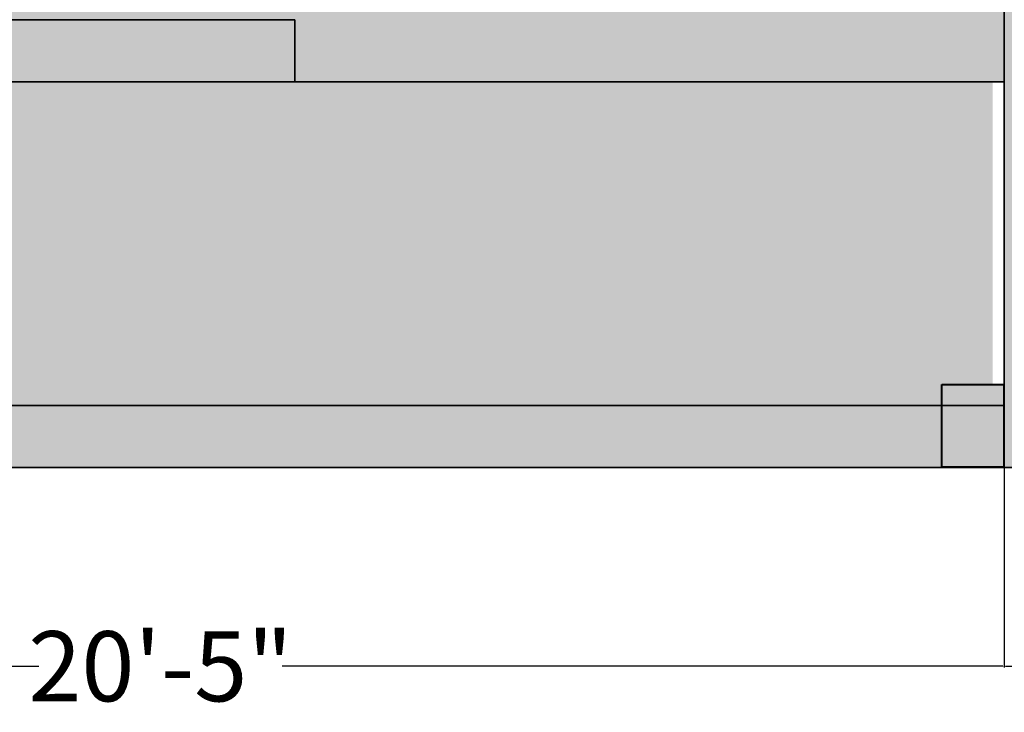
# Model space of a CAD drawing. Units: inches. Extents: x 1077 to 2505, y 1892 to 2728.
# Tile 4 of 26: x 1290 to 1433, y 2053 to 2153. Entities that reach past the tile are written whole.
import ezdxf

# ---------------------------------------------------------------- set-up
doc = ezdxf.new("R2010")
doc.units = ezdxf.units.IN
doc.linetypes.add('ACAD_ISO02W100', pattern=[15, 12, -3])
doc.layers.get('Defpoints').update_dxf_attribs({"color": 220, "linetype": 'ACAD_ISO02W100'})
for name, color, linetype, lineweight in [('A-ANNO-DIMS', 2, 'Continuous', 18), ('A-COLS', 7, 'Continuous', 40), ('A-WALL-PATT', 7, 'Continuous', 9), ('WALL', 7, 'Continuous', 35)]:
    doc.layers.add(name, color=color, linetype=linetype, lineweight=lineweight)
doc.layers.add('A-FLOR-PATT', color=254, linetype='Continuous', lineweight=9, true_color=0xd7ebd2)
doc.layers.add('L-PLNT-PATT', color=116, linetype='Continuous', lineweight=9, true_color=0x136734)
doc.styles.get("Standard").update_dxf_attribs({"font": 'arial.ttf'})
doc.dimstyles.get("Standard").update_dxf_attribs({"dimtxt": 10.18, "dimasz": 0.18, "dimexe": 0.18, "dimexo": 0.0625, "dimgap": 0.09, "dimtad": 0, "dimtih": 1, "dimtoh": 1, "dimdec": 0, "dimzin": 0, "dimdsep": 46, "dimlunit": 3, "dimtxsty": 'Standard', "dimcen": 0.09, "dimadec": 0, "dimazin": 0, "dimtfac": 1, "dimtdec": 0, "dimtofl": 0, "dimtmove": 0, "dimatfit": 3, "dimfxl": 1, "dimtolj": 1, "dimtzin": 0, "dimarcsym": 0})

# ---------------------------------------------------------------- blocks, each defined once
blk = doc.blocks.new('C1')
h = blk.add_hatch(color=256)
h.dxf.hatch_style = 1
h.paths.add_polyline_path([(1668.56, 2445.41), (1677.56, 2445.41), (1677.56, 2457.41), (1668.56, 2457.41)])
for p, q in [((1668.56, 2457.41), (1677.56, 2457.41)), ((1668.56, 2445.41), (1668.56, 2457.41)), ((1677.56, 2457.41), (1677.56, 2445.41)), ((1677.56, 2445.41), (1668.56, 2445.41))]:
    blk.add_line(p, q)
blk = doc.blocks.new('*D65')
at = {"layer": 'A-ANNO-DIMS', "color": 0, "lineweight": -2, "transparency": 16777216}
for p, q in [((1187.53, 2097.1), (1187.53, 2059.13)), ((1432.53, 2097.1), (1432.53, 2059.13)), ((1187.71, 2059.31), (1292.37, 2059.31)), ((1432.35, 2059.31), (1327.69, 2059.31))]:
    blk.add_line(p, q, dxfattribs=at)
at = {"layer": 'A-ANNO-DIMS', "color": 0, "transparency": 16777216}
for points in [[(1187.71, 2059.34), (1187.71, 2059.28), (1187.53, 2059.31)], [(1432.35, 2059.34), (1432.35, 2059.28), (1432.53, 2059.31)]]:
    blk.add_solid(points, dxfattribs=at)
at = {"layer": 'Defpoints', "color": 0, "transparency": 16777216}
for p in [(1187.53, 2097.16), (1432.53, 2097.16), (1432.53, 2059.31)]:
    blk.add_point(p, dxfattribs=at)
at = {"layer": 'A-ANNO-DIMS', "color": 0, "transparency": 16777216, "insert": (1310.03, 2059.31), "char_height": 10.18, "attachment_point": 5}
blk.add_mtext('\\A1;20\'-5"', dxfattribs=at)
blk = doc.blocks.new('*D67')
at = {"layer": 'A-ANNO-DIMS', "color": 0, "lineweight": -2, "transparency": 16777216}
for p, q in [((1432.53, 2088.1), (1432.53, 2059.13)), ((1547.53, 2088.1), (1547.53, 2059.13)), ((1432.71, 2059.31), (1476.41, 2059.31)), ((1547.35, 2059.31), (1503.65, 2059.31))]:
    blk.add_line(p, q, dxfattribs=at)
at = {"layer": 'A-ANNO-DIMS', "color": 0, "transparency": 16777216}
for points in [[(1432.71, 2059.34), (1432.71, 2059.28), (1432.53, 2059.31)], [(1547.35, 2059.34), (1547.35, 2059.28), (1547.53, 2059.31)]]:
    blk.add_solid(points, dxfattribs=at)
at = {"layer": 'Defpoints', "color": 0, "transparency": 16777216}
for p in [(1432.53, 2088.16), (1547.53, 2088.16), (1547.53, 2059.31)]:
    blk.add_point(p, dxfattribs=at)
at = {"layer": 'A-ANNO-DIMS', "color": 0, "transparency": 16777216, "insert": (1490.03, 2059.31), "char_height": 10.18, "attachment_point": 5}
blk.add_mtext('\\A1;9\'-7"', dxfattribs=at)

msp = doc.modelspace()

# ---------------------------------------------------------------- hatches: boundary and pattern name
at = {"layer": 'A-FLOR-PATT', "transparency": 33554559}
h = msp.add_hatch(color=256, dxfattribs=at)
h.dxf.hatch_style = 1
h.paths.add_polyline_path([(1395.53, 2577.16), (1374.83, 2577.16), (1350.83, 2577.19), (1350.83, 2577.16), (1329.53, 2577.16), (1329.53, 2480.16), (1329.53, 2469.16), (1325.53, 2469.16), (1325.53, 2515.13), (1307.53, 2515.13), (1307.53, 2577.16), (1269.31, 2577.16), (1221.31, 2577.15), (1221.31, 2577.16), (1187.53, 2577.16), (1187.53, 2433.16), (1289.53, 2433.16), (1289.53, 2429.16), (1263.53, 2429.16), (1187.53, 2429.16), (1187.53, 2395.02), (1187.53, 2395.02), (1187.53, 2371.02), (1187.53, 2371.02), (1187.53, 2307.16), (1259.53, 2307.16), (1259.53, 2399.16), (1263.53, 2399.16), (1263.53, 2307.16), (1289.53, 2307.16), (1289.53, 2306.23), (1325.53, 2306.23), (1325.53, 2307.16), (1329.53, 2307.16), (1329.53, 2306.23), (1365.53, 2306.23), (1365.53, 2307.16), (1432.53, 2307.16), (1432.53, 2088.16), (1547.53, 2088.16), (1547.53, 2140.08), (1511.53, 2140.08), (1511.53, 2267.16), (1475.53, 2267.16), (1475.53, 2303.16), (1468.53, 2303.16), (1468.53, 2307.16), (1547.53, 2307.16), (1547.53, 2348.22), (1547.53, 2396.22), (1547.53, 2429.16), (1435.53, 2429.16), (1435.53, 2433.16), (1476.35, 2433.16), (1476.35, 2451.18), (1547.53, 2451.18), (1547.53, 2577.16), (1499.53, 2577.16), (1499.53, 2586.16), (1547.53, 2586.16), (1547.53, 2642.16), (1518.18, 2642.16), (1518.18, 2642.05), (1494.15, 2642.05), (1494.15, 2642.16), (1469.53, 2642.16), (1469.53, 2577.16), (1399.53, 2577.16), (1399.53, 2429.16), (1325.53, 2429.16), (1325.53, 2433.16), (1329.53, 2433.16), (1395.53, 2433.16), (1395.53, 2480.16), (1359.53, 2480.16), (1359.53, 2484.16), (1395.53, 2484.16)])
h.paths.add_polyline_path([(1357.65, 2482.07), (1355.65, 2482.07), (1355.65, 2481.07, 0.414214), (1356.65, 2480.07), (1344.65, 2480.07), (1344.65, 2477.06), (1343.27, 2477.06), (1343.27, 2480.07), (1330.65, 2480.07, -0.414214), (1329.65, 2481.07), (1329.65, 2484.07), (1331.65, 2484.07), (1331.65, 2510.07, -0.446908)], flags=16)
h.paths.add_polyline_path([(1305.09, 2559.18), (1288.89, 2559.18), (1288.89, 2575.38), (1305.09, 2575.38)], flags=16)
h.paths.add_polyline_path([(1304.19, 2560.08), (1289.79, 2560.08), (1289.79, 2574.48), (1304.19, 2574.48)], flags=0)
h.paths.add_polyline_path([(1287.99, 2500.68, -0.414214), (1287.09, 2499.78), (1265.14, 2499.78), (1224.09, 2499.78, -0.414214), (1223.19, 2500.68), (1223.19, 2557.16), (1223.19, 2571.74), (1223.19, 2575.38), (1287.99, 2575.38), (1287.99, 2571.74), (1287.09, 2571.74, -0.414214), (1287.99, 2570.84)], flags=16)
h.paths.add_polyline_path([(1292.98, 2569.05, -1), (1300.92, 2569.05, -1)], flags=0)
h.paths.add_polyline_path([(1293.32, 2569.05, -1), (1300.58, 2569.05, -1)], flags=0)
h.paths.add_polyline_path([(1322.8, 2462.21), (1322.8, 2431.71), (1323.05, 2430.71), (1323.05, 2431.71), (1321.8, 2431.71), (1321.8, 2462.19, 0.404641), (1292.3, 2431.71), (1292.05, 2430.71, -0.414214), (1291.55, 2430.21), (1291.05, 2430.21), (1291.05, 2429.71, -0.414214), (1290.55, 2429.21), (1289.55, 2429.21), (1289.55, 2434.21), (1290.55, 2434.21, -0.414214), (1291.05, 2433.71), (1291.05, 2433.21), (1291.55, 2433.21, -0.414214), (1292.05, 2432.71), (1292.3, 2431.71, -0.414214)], flags=16)
h.paths.add_polyline_path([(1287.82, 2548.28, 0.292232), (1279.17, 2536.8, 0.052719), (1223.93, 2548.28), (1223.28, 2548.28), (1223.28, 2557.16), (1223.93, 2557.16), (1245.42, 2557.16, -0.117785), (1245.77, 2557.93, -0.059418), (1254.87, 2567.02, -0.379859), (1257.28, 2566.88, -0.02509), (1261.41, 2563.32, -0.025935), (1265.65, 2567.02, -0.379859), (1268.06, 2566.88, -0.061767), (1277.52, 2557.43, -0.069393), (1277.82, 2557.16), (1287.82, 2557.16)], flags=0)
h.paths.add_polyline_path([(1263.47, 2548.28), (1260.56, 2548.28, -0.015371), (1258.01, 2546.13, -0.429576), (1255.37, 2546.06, -0.016036), (1252.69, 2548.28), (1223.28, 2548.28), (1223.28, 2554.42), (1246.78, 2554.42, 0.055344), (1255.37, 2546.06, 0.331768), (1257.52, 2545.74, 0.027343), (1262, 2549.64, 0.00919)], flags=0)
h.paths.add_polyline_path([(1295.56, 2568.34), (1296.87, 2569.09), (1296.87, 2570.6, 0.399698), (1295.39, 2569.05, 0.119004)], flags=0)
h.paths.add_polyline_path([(1295.21, 2569.05, -1), (1298.68, 2569.05, -1)], flags=0)
h.paths.add_polyline_path([(1296.95, 2568.96), (1297.03, 2569), (1297.03, 2569.09), (1296.99, 2569.11), (1296.91, 2568.98)], flags=0)
h.paths.add_polyline_path([(1402.28, 2462.19, -0.414214), (1432.78, 2431.69), (1433.03, 2432.69), (1432.78, 2431.69, 0.404641), (1403.28, 2462.17), (1403.28, 2431.69), (1402.03, 2431.69), (1402.03, 2430.69, -0.414214), (1401.53, 2430.19), (1401.03, 2430.19), (1401.03, 2429.69, -0.414214), (1400.53, 2429.19), (1399.53, 2429.19), (1399.53, 2434.19), (1400.53, 2434.19, -0.414214), (1401.03, 2433.69), (1401.03, 2433.19), (1401.53, 2433.19, -0.414214), (1402.03, 2432.69)], flags=16)
h.paths.add_polyline_path([(1470.16, 2535.21, -0.414214), (1471.06, 2536.11), (1527.54, 2536.11), (1542.12, 2536.11), (1545.76, 2536.11), (1545.76, 2471.31), (1542.12, 2471.31), (1542.12, 2472.21, -0.414214), (1541.22, 2471.31), (1471.06, 2471.31, -0.414214), (1470.16, 2472.21), (1470.16, 2494.16)], flags=16)
h.paths.add_polyline_path([(1483.07, 2536.11, 0.253465), (1480.11, 2526.15, 0.2538), (1470.15, 2523.19)], flags=16)
h.paths.add_polyline_path([(1223.19, 2512.69, 0.253465), (1233.14, 2509.74, 0.2538), (1236.1, 2499.77)], flags=16)
h.paths.add_polyline_path([(1469.77, 2578.72), (1469.77, 2581.72), (1471.77, 2581.72), (1471.77, 2607.72, -0.01951), (1473.77, 2607.68), (1473.77, 2579.72), (1473.77, 2578.72, -0.414214), (1472.77, 2577.72), (1470.77, 2577.72, -0.414214)], flags=16)
h.paths.add_polyline_path([(1382.46, 2398.13), (1395.04, 2398.13), (1395.04, 2399.74), (1382.46, 2399.74)], flags=16)
h.paths.add_polyline_path([(1379.94, 2397.18), (1379.94, 2389.82), (1380.5, 2389.82), (1380.5, 2396.05, -0.41429), (1381.06, 2396.61), (1396.47, 2396.61, -0.414213), (1397.03, 2396.05), (1397.03, 2389.82), (1397.59, 2389.82), (1397.59, 2397.18)], flags=16)
h.paths.add_polyline_path([(1263.37, 2428.14), (1263.37, 2426.14, -0.414214), (1262.37, 2425.14), (1261.37, 2425.14), (1233.41, 2425.14, 0.400854), (1259.37, 2401.04), (1259.37, 2401.14), (1261.37, 2401.14, -0.446908), (1233.37, 2427.14), (1259.37, 2427.14), (1259.37, 2429.14), (1262.37, 2429.14, -0.414214)], flags=16)
h.paths.add_polyline_path([(1404.79, 2398.13), (1417.37, 2398.13), (1417.37, 2399.74), (1404.79, 2399.74)], flags=16)
h.paths.add_polyline_path([(1402.27, 2397.18), (1404.79, 2398.13), (1417.37, 2398.13), (1419.92, 2397.18)], flags=16)
h.paths.add_polyline_path([(1432.26, 2383.16), (1432.26, 2370.59), (1433.87, 2370.59), (1433.87, 2383.16)], flags=16)
h.paths.add_polyline_path([(1431.3, 2385.69), (1423.84, 2385.69), (1423.84, 2385.13), (1430.18, 2385.13, -0.41429), (1430.74, 2384.57), (1430.74, 2369.16, -0.414237), (1430.18, 2368.6), (1423.84, 2368.6), (1423.84, 2368.03), (1431.3, 2368.03)], flags=16)
h.paths.add_polyline_path([(1417.37, 2351.16), (1417.37, 2349.54), (1418.9, 2349.54, 0.414236), (1419.92, 2350.56), (1419.92, 2352.11)], flags=16)
h.paths.add_polyline_path([(1395.04, 2351.16), (1395.04, 2349.54), (1396.58, 2349.54, 0.414235), (1397.59, 2350.56), (1397.59, 2352.11)], flags=16)
h.paths.add_polyline_path([(1366.7, 2370.05), (1365.09, 2370.05), (1365.09, 2368.52, 0.414235), (1366.11, 2367.5), (1367.66, 2367.5)], flags=16)
h.paths.add_polyline_path([(1419.36, 2359.47), (1419.36, 2353.24, -0.41419), (1418.8, 2352.68), (1403.39, 2352.68, -0.414137), (1402.83, 2353.24), (1402.83, 2359.47), (1397.03, 2359.47), (1397.03, 2353.24, -0.414189), (1396.47, 2352.68), (1381.06, 2352.68, -0.414137), (1380.5, 2353.24), (1380.5, 2359.47)], flags=16)
h.paths.add_polyline_path([(1222.29, 2559.18), (1206.09, 2559.18), (1206.09, 2575.38), (1222.29, 2575.38)], flags=16)
h.paths.add_polyline_path([(1221.39, 2560.08), (1206.99, 2560.08), (1206.99, 2574.48), (1221.39, 2574.48)], flags=0)
h.paths.add_polyline_path([(1482, 2577.72), (1482, 2580.73), (1483.38, 2580.73), (1483.38, 2577.72), (1484.77, 2577.72), (1484.77, 2574.72), (1483.38, 2574.72), (1483.38, 2577.72)], flags=16)
h.paths.add_polyline_path([(1266.37, 2415.53), (1266.37, 2414.14), (1263.37, 2414.14), (1263.37, 2415.53), (1260.36, 2415.53), (1260.36, 2416.91), (1263.37, 2416.91), (1263.37, 2415.53)], flags=16)
h.paths.add_polyline_path([(1210.26, 2569.05, -1), (1218.19, 2569.05, -1)], flags=0)
h.paths.add_polyline_path([(1210.6, 2569.05, -1), (1217.85, 2569.05, -1)], flags=0)
h.paths.add_polyline_path([(1212.84, 2568.34), (1214.15, 2569.09), (1214.15, 2570.6, 0.399698), (1212.67, 2569.05, 0.119004)], flags=0)
h.paths.add_polyline_path([(1212.49, 2569.05, -1), (1215.96, 2569.05, -1)], flags=0)
h.paths.add_polyline_path([(1214.23, 2568.96), (1214.3, 2568.91), (1214.3, 2569)], flags=0)
h.paths.add_polyline_path([(1507.18, 2480.12, 0.052719), (1518.66, 2535.36), (1518.66, 2536.01), (1527.54, 2536.01), (1527.54, 2535.36), (1527.54, 2513.88, -0.117785), (1528.31, 2513.53, -0.059418), (1537.4, 2504.43, -0.379859), (1537.26, 2502.01, -0.02509), (1533.7, 2497.89, -0.025935), (1537.4, 2493.64, -0.379859), (1537.26, 2491.23, -0.061767), (1527.8, 2481.77, -0.069393), (1527.54, 2481.47), (1527.54, 2471.47), (1518.66, 2471.47, 0.292232)], flags=0)
h.paths.add_polyline_path([(1516.43, 2503.92, -0.016036), (1518.66, 2506.6), (1518.66, 2536.01), (1524.8, 2536.01), (1524.8, 2512.51, 0.055344), (1516.43, 2503.92, 0.331768), (1516.12, 2501.77, 0.027343), (1520.01, 2497.29, 0.00919), (1518.66, 2495.82), (1518.66, 2498.73, -0.015371), (1516.5, 2501.28, -0.429576)], flags=0)
h.paths.add_polyline_path([(1499.63, 2625.5, -0.171636), (1502.82, 2631.01), (1502.82, 2633.37), (1498.68, 2633.37, -0.414214), (1497.7, 2634.36), (1497.7, 2640.66, -0.414214), (1498.68, 2641.64), (1514.82, 2641.64, -0.414214), (1515.81, 2640.66), (1515.81, 2634.36, -0.414214), (1514.82, 2633.37), (1510.69, 2633.37), (1510.69, 2631.01, -0.171636), (1513.88, 2625.5, -0.258205), (1509.31, 2614.47), (1504.19, 2614.47, -0.258205)], flags=16)
h.paths.add_polyline_path([(1501.2, 2625.5, -0.171636), (1504.39, 2631.01), (1509.12, 2631.01, -0.171636), (1512.3, 2625.5, -0.210384), (1509.35, 2616.02), (1504.16, 2616.02, -0.210384)], flags=0)
h.paths.add_polyline_path([(1529.56, 2537.01), (1529.56, 2553.21), (1545.76, 2553.21), (1545.76, 2537.01)], flags=16)
h.paths.add_polyline_path([(1530.46, 2537.91), (1530.46, 2552.31), (1544.86, 2552.31), (1544.86, 2537.91)], flags=0)
h.paths.add_polyline_path([(1535.45, 2545.07, -1), (1543.39, 2545.07, -1)], flags=0)
h.paths.add_polyline_path([(1535.8, 2545.07, -1), (1543.05, 2545.07, -1)], flags=0)
h.paths.add_polyline_path([(1529.56, 2470.41), (1545.76, 2470.41), (1545.76, 2454.21), (1529.56, 2454.21)], flags=16)
h.paths.add_polyline_path([(1541.16, 2544.99), (1540.98, 2544.99, -0.544606), (1538.71, 2543.68), (1538.62, 2543.53, 0.547962)], flags=0)
h.paths.add_polyline_path([(1530.46, 2469.51), (1544.86, 2469.51), (1544.86, 2455.11), (1530.46, 2455.11)], flags=0)
h.paths.add_polyline_path([(1539.47, 2545.14), (1539.42, 2545.22), (1539.38, 2545.14)], flags=0)
h.paths.add_polyline_path([(1543.39, 2462.34, -1), (1535.45, 2462.34, -1)], flags=0)
h.paths.add_polyline_path([(1543.05, 2462.34, -1), (1535.8, 2462.34, -1)], flags=0)
h.paths.add_polyline_path([(1541.16, 2462.27), (1540.98, 2462.27, -0.544606), (1538.71, 2460.96), (1538.62, 2460.8, 0.547962)], flags=0)
h.paths.add_polyline_path([(1539.47, 2462.42), (1539.42, 2462.5), (1539.38, 2462.42)], flags=0)
h.paths.add_polyline_path([(1435.32, 2335.25, -0.414214), (1465.82, 2304.75), (1466.07, 2305.75), (1465.82, 2304.75, 0.404641), (1436.32, 2335.23), (1436.32, 2304.75), (1435.07, 2304.75), (1435.07, 2303.75, -0.414214), (1434.57, 2303.25), (1434.07, 2303.25), (1434.07, 2302.75, -0.414214), (1433.57, 2302.25), (1432.57, 2302.25), (1432.57, 2307.25), (1433.57, 2307.25, -0.414214), (1434.07, 2306.75), (1434.07, 2306.25), (1434.57, 2306.25, -0.414214), (1435.07, 2305.75)], flags=16)
h.paths.add_polyline_path([(1532.13, 2635.71), (1535.43, 2635.71), (1535.43, 2635.89), (1532.13, 2635.89)], flags=16)
edge = h.paths.add_edge_path(flags=16)
edge.add_arc((1535.98, 2632.67), 0.183, 270, 360)
edge.add_line((1536.17, 2632.67), (1536.17, 2639.82))
edge.add_line((1536.17, 2639.82), (1538.29, 2639.82))
edge.add_line((1538.29, 2639.82), (1538.29, 2641.82))
edge.add_line((1538.29, 2641.82), (1533.25, 2641.82))
edge.add_line((1533.25, 2641.82), (1533.25, 2639.82))
edge.add_line((1533.25, 2639.82), (1534.87, 2639.82))
edge.add_line((1534.87, 2639.82), (1534.87, 2639))
edge.add_line((1534.87, 2639), (1533.7, 2639))
edge.add_line((1533.7, 2639), (1533.7, 2639.82))
edge.add_line((1533.7, 2639.82), (1533.25, 2639.82))
edge.add_line((1533.25, 2639.82), (1533.25, 2641.82))
edge.add_line((1533.25, 2641.82), (1538.29, 2641.82))
edge.add_line((1538.29, 2641.82), (1538.29, 2641.34))
edge.add_line((1538.29, 2641.34), (1540.64, 2641.58))
edge.add_line((1540.64, 2641.58), (1540.64, 2641.82))
edge.add_line((1540.64, 2641.82), (1541.5, 2641.82))
edge.add_line((1541.5, 2641.82), (1541.5, 2641.25))
edge.add_line((1541.5, 2641.25), (1541.31, 2639.79))
edge.add_ellipse((1541.09, 2638.95), major_axis=(-1.08, 0), ratio=0.790849, start_angle=180, end_angle=255.2976, ccw=False)
edge.add_line((1542.17, 2638.95), (1542.17, 2638.38))
edge.add_ellipse((1541.09, 2638.38), major_axis=(-1.08, 0), ratio=0.790849, start_angle=0, end_angle=180, ccw=False)
edge.add_line((1540, 2638.38), (1540.01, 2638.87))
edge.add_ellipse((1541.09, 2638.95), major_axis=(-1.08, 0), ratio=0.790849, start_angle=284.7024, end_angle=364.0401, ccw=False)
edge.add_line((1540.78, 2639.75), (1540.78, 2641.25))
edge.add_line((1540.78, 2641.25), (1540.64, 2641.25))
edge.add_line((1540.64, 2641.25), (1538.29, 2641.01))
edge.add_line((1538.29, 2641.01), (1538.29, 2639.82))
edge.add_line((1538.29, 2639.82), (1536.17, 2639.82))
edge.add_line((1536.17, 2639.82), (1536.17, 2632.48))
edge.add_line((1536.17, 2632.48), (1535.98, 2632.48))
h.paths.add_polyline_path([(1496.32, 2250.34, -0.292371), (1498.9, 2247.83, -0.085148), (1501.21, 2208.85, -0.01331), (1500.27, 2098.5, -0.379287), (1497.22, 2095.28, -0.0502), (1441.54, 2095.28, -0.379287), (1438.5, 2098.5, -0.01331), (1437.56, 2208.85, -0.086132), (1439.96, 2248.26, -0.295116), (1442.59, 2250.78, -0.114238)], flags=16)
h.paths.add_polyline_path([(1495.16, 2205.84, -0.355389), (1496.7, 2202.1), (1492.94, 2189.65, -0.398275), (1489.12, 2187.47, 0.113332), (1449.64, 2187.47, -0.398275), (1445.82, 2189.65), (1442.06, 2202.1, -0.355394), (1443.6, 2205.84, -0.265725)], flags=0)
h.paths.add_polyline_path([(1440.37, 2195.72), (1445.94, 2181.67), (1445.94, 2160.63), (1440.84, 2157.26)], flags=0)
h.paths.add_polyline_path([(1498.46, 2195.72), (1497.99, 2157.26), (1492.88, 2160.63), (1492.88, 2181.67)], flags=0)
h.paths.add_polyline_path([(1445.94, 2158.37), (1445.94, 2137.12), (1441.12, 2122.56), (1440.87, 2155.03)], flags=0)
h.paths.add_polyline_path([(1492.88, 2158.37), (1497.96, 2155.03), (1497.71, 2122.56), (1492.88, 2137.12)], flags=0)
h.paths.add_polyline_path([(1489.88, 2130.4), (1494.39, 2107.67, -0.090102), (1444.44, 2107.65), (1448.95, 2130.39, 0.036636)], flags=0)
h.paths.add_polyline_path([(1447.54, 2159.34), (1497.44, 2159.34), (1497.44, 2177.89), (1447.54, 2177.89)], flags=8)
h.paths.add_polyline_path([(1196.44, 2354.84), (1246.65, 2354.84), (1246.65, 2388.43), (1196.44, 2388.43)], flags=24)
h.paths.add_polyline_path([(1296.09, 2360.25), (1353.81, 2360.25), (1353.81, 2393.84), (1296.09, 2393.84)], flags=24)
h.paths.add_polyline_path([(1400.72, 2471.85), (1470.63, 2471.85), (1470.63, 2505.44), (1400.72, 2505.44)], flags=24)
h.paths.add_polyline_path([(1324.78, 2448.48), (1394.95, 2448.48), (1394.95, 2467.02), (1324.78, 2467.02)], flags=24)
h.paths.add_polyline_path([(1335.08, 2531.43), (1389.67, 2531.43), (1389.67, 2565.02), (1335.08, 2565.02)], flags=24)
h.paths.add_polyline_path([(1225.76, 2460), (1295.67, 2460), (1295.67, 2493.58), (1225.76, 2493.58)], flags=24)
h = msp.add_hatch(color=256, dxfattribs=at)
h.dxf.hatch_style = 1
h.paths.add_polyline_path([(1547.53, 2348.22), (1547.53, 2396.22), (1547.53, 2425.11), (1547.53, 2425.11), (1547.53, 2429.16), (1435.53, 2429.16), (1434.03, 2429.21), (1434.03, 2430.19), (1433.03, 2430.19), (1432.78, 2431.69, 0.404641), (1403.28, 2462.17), (1403.28, 2431.69), (1402.03, 2431.69), (1402.03, 2430.19), (1401.03, 2430.19), (1401.03, 2429.19), (1399.53, 2429.19), (1399.53, 2429.19), (1399.53, 2429.16), (1334.67, 2429.16), (1334.67, 2423.95), (1325.67, 2423.95), (1325.67, 2429.16), (1325.53, 2429.16), (1324.05, 2429.24), (1324.05, 2430.21), (1323.05, 2430.21), (1323.05, 2431.71), (1321.8, 2431.71), (1321.8, 2462.19, 0.416544), (1292.05, 2430.73, -0.423614), (1291.55, 2430.21), (1291.05, 2430.21), (1291.05, 2429.21), (1289.55, 2429.21), (1289.53, 2429.21), (1289.53, 2429.16), (1263.37, 2429.16), (1263.37, 2415.53), (1266.37, 2415.53), (1266.37, 2414.14), (1263.37, 2414.14), (1263.37, 2399.16), (1263.53, 2399.16), (1263.53, 2307.16), (1289.53, 2307.16), (1289.53, 2306.23), (1323.26, 2306.23), (1323.26, 2307.21), (1332.26, 2307.21), (1365.53, 2306.23), (1365.53, 2307.16), (1432.53, 2307.16), (1432.57, 2307.16), (1432.57, 2307.25), (1434.07, 2307.25), (1434.07, 2306.25), (1435.32, 2306.25), (1435.32, 2335.25, -0.407346), (1466.07, 2305.73, -0.423614), (1466.57, 2306.25), (1467.07, 2306.25), (1467.07, 2307.25), (1468.57, 2307.25), (1547.53, 2307.16), (1547.53, 2307.2)])
h.paths.add_polyline_path([(1430.74, 2369.16), (1430.74, 2384.57, 0.41429), (1430.18, 2385.13), (1423.84, 2385.13), (1423.84, 2368.6), (1430.18, 2368.6, 0.414237)], flags=16)
h.paths.add_polyline_path([(1432.26, 2383.16), (1432.26, 2370.59), (1433.87, 2370.59), (1433.87, 2383.16)], flags=16)
h.paths.add_polyline_path([(1431.3, 2368.03), (1431.3, 2385.69), (1432.26, 2383.16), (1432.26, 2370.59)], flags=16)
h.paths.add_polyline_path([(1417.37, 2351.16), (1417.37, 2349.54), (1418.9, 2349.54, 0.414236), (1419.92, 2350.56), (1419.92, 2352.11)], flags=16)
h.paths.add_polyline_path([(1403.39, 2352.68), (1418.78, 2352.68, 0.42427), (1419.36, 2353.24), (1419.36, 2359.47), (1402.83, 2359.47), (1402.83, 2353.24, 0.414137)], flags=16)
h.paths.add_polyline_path([(1366.7, 2370.05), (1365.09, 2370.05), (1365.09, 2368.52, 0.414235), (1366.11, 2367.5), (1367.66, 2367.5)], flags=16)
h.paths.add_polyline_path([(1382.46, 2398.13), (1395.04, 2398.13), (1395.04, 2399.74), (1382.46, 2399.74)], flags=16)
h.paths.add_polyline_path([(1396.47, 2396.61), (1381.06, 2396.61, 0.41429), (1380.5, 2396.05), (1380.5, 2389.82), (1397.03, 2389.82), (1397.03, 2396.05, 0.414213)], flags=16)
h.paths.add_polyline_path([(1402.27, 2397.18), (1402.83, 2396.05, -0.414213), (1403.39, 2396.61)], flags=16)
h.paths.add_polyline_path([(1418.8, 2396.61), (1419.36, 2396.61), (1419.36, 2396.05, 0.414237)], flags=16)
h.paths.add_polyline_path([(1404.79, 2398.13), (1417.37, 2398.13), (1417.37, 2399.74), (1404.79, 2399.74)], flags=16)
h.paths.add_polyline_path([(1381.06, 2352.68, -0.414213), (1380.5, 2353.24), (1380.27, 2352.11)], flags=16)
h.paths.add_polyline_path([(1396.58, 2349.54), (1396.58, 2349.54), (1395.04, 2349.54), (1395.04, 2349.54), (1382.46, 2349.54), (1382.46, 2351.16), (1395.04, 2351.16), (1397.59, 2352.11), (1397.59, 2350.56, -0.414235)], flags=16)
h.paths.add_polyline_path([(1379.94, 2397.18), (1382.46, 2398.13), (1395.04, 2398.13), (1397.59, 2397.18)], flags=16)
h.paths.add_polyline_path([(1368.78, 2384.59, 0.414213), (1368.22, 2384.03), (1367.66, 2367.5), (1367.66, 2385.15)], flags=16)
h.paths.add_polyline_path([(1547.53, 2574.38), (1547.51, 2574.38), (1547.51, 2577.16), (1499.53, 2577.16), (1484.77, 2577.44), (1484.77, 2574.72), (1483.38, 2574.72), (1483.38, 2577.72), (1482, 2577.72), (1469.53, 2577.72), (1469.53, 2577.16), (1401.95, 2577.16), (1401.95, 2574.12), (1399.53, 2574.12), (1399.53, 2434.19), (1401.03, 2434.19), (1401.03, 2433.19), (1402.28, 2433.19), (1402.28, 2462.19, -0.407346), (1433.03, 2432.67, -0.423614), (1433.53, 2433.19), (1434.03, 2433.19), (1434.03, 2434.19), (1435.53, 2434.19), (1476.35, 2433.81), (1476.35, 2451.18), (1547.53, 2451.18)])
h.paths.add_polyline_path([(1470.16, 2535.21, -0.414214), (1471.06, 2536.11), (1527.54, 2536.11), (1542.12, 2536.11), (1545.76, 2536.11), (1545.76, 2471.31), (1542.12, 2471.31), (1542.12, 2472.21, -0.414214), (1541.22, 2471.31), (1471.06, 2471.31, -0.414214), (1470.16, 2472.21), (1470.16, 2494.16)], flags=16)
h.paths.add_polyline_path([(1483.07, 2536.11, 0.253465), (1480.11, 2526.15, 0.2538), (1470.15, 2523.19)], flags=16)
h.paths.add_polyline_path([(1525.55, 2481.52, -0.000893), (1524.8, 2482.24), (1524.8, 2471.47), (1527.54, 2471.47), (1527.54, 2472.12), (1527.54, 2481.47, -0.388819)], flags=0)
h.paths.add_polyline_path([(1518.66, 2536.01), (1527.54, 2536.01), (1527.54, 2535.36), (1527.54, 2513.88, -0.117785), (1528.31, 2513.53, -0.059418), (1537.4, 2504.43, -0.379859), (1537.26, 2502.01, -0.02509), (1533.7, 2497.89, 0.033431), (1528.3, 2502.74, 0.308459), (1526.25, 2502.88, 0.047827), (1518.66, 2495.82), (1518.66, 2498.73, -0.015371), (1516.5, 2501.28, -0.429576), (1516.43, 2503.92, -0.016036), (1518.66, 2506.6)], flags=0)
h.paths.add_polyline_path([(1529.56, 2537.01), (1529.56, 2553.21), (1545.76, 2553.21), (1545.76, 2537.01)], flags=16)
h.paths.add_polyline_path([(1530.46, 2537.91), (1530.46, 2552.31), (1544.86, 2552.31), (1544.86, 2537.91)], flags=0)
h.paths.add_polyline_path([(1535.8, 2545.07, -1), (1543.05, 2545.07, -1)], flags=0)
h.paths.add_polyline_path([(1541.16, 2544.99), (1540.98, 2544.99, -0.544606), (1538.71, 2543.68), (1538.62, 2543.53, 0.547962)], flags=0)
h.paths.add_polyline_path([(1539.47, 2545.14), (1539.42, 2545.22), (1539.38, 2545.14)], flags=0)
h.paths.add_polyline_path([(1529.56, 2470.41), (1545.76, 2470.41), (1545.76, 2454.21), (1529.56, 2454.21)], flags=16)
h.paths.add_polyline_path([(1530.46, 2469.51), (1544.86, 2469.51), (1544.86, 2455.11), (1530.46, 2455.11)], flags=0)
h.paths.add_polyline_path([(1535.8, 2462.34, -1), (1543.05, 2462.34, -1)], flags=0)
h.paths.add_polyline_path([(1541.16, 2462.27), (1540.98, 2462.27, -0.544606), (1538.71, 2460.96), (1538.62, 2460.8, 0.547962)], flags=0)
h.paths.add_polyline_path([(1539.47, 2462.42), (1539.42, 2462.5), (1539.38, 2462.42)], flags=0)
h.paths.add_polyline_path([(1395.53, 2574.12), (1392.95, 2574.12), (1392.95, 2577.16), (1374.83, 2577.16), (1350.83, 2577.19), (1350.83, 2577.16), (1332.07, 2577.16), (1332.07, 2574), (1329.53, 2574), (1329.53, 2484.07), (1331.65, 2484.07), (1331.65, 2510.07, -0.423677), (1357.76, 2484.07), (1359.53, 2484.07), (1359.53, 2484.16), (1395.53, 2484.16)], flags=17)
h.paths.add_polyline_path([(1395.53, 2480.16), (1359.06, 2480.16, 0.437533), (1359.53, 2481.55), (1359.53, 2484.16), (1395.53, 2484.16), (1395.53, 2574.12), (1392.95, 2574.12), (1392.95, 2577.16), (1374.83, 2577.16), (1350.83, 2577.19), (1350.83, 2577.16), (1332.07, 2577.16), (1332.07, 2574), (1329.53, 2574), (1329.53, 2484.07), (1329.65, 2484.07), (1329.65, 2481.07), (1329.53, 2480.16), (1329.53, 2469.16), (1325.53, 2469.16), (1325.53, 2515.13), (1307.53, 2515.13), (1307.53, 2577.16), (1269.31, 2577.16), (1221.31, 2577.15), (1221.31, 2577.16), (1187.61, 2577.16), (1187.61, 2574.03), (1187.53, 2433.16), (1289.55, 2433.16), (1289.55, 2434.21), (1291.05, 2434.21), (1291.05, 2433.21), (1292.05, 2433.21), (1292.3, 2431.71, -0.414214), (1322.8, 2462.21), (1323.05, 2432.71, -0.414214), (1323.55, 2433.21), (1324.05, 2433.21), (1324.05, 2434.21), (1325.67, 2434.21), (1325.67, 2435.95), (1334.67, 2435.95), (1334.67, 2433.16), (1395.53, 2433.16)])
h.paths.add_polyline_path([(1344.65, 2480.07), (1344.65, 2477.06), (1343.27, 2477.06), (1343.27, 2480.07), (1332.65, 2480.07, 0.414214), (1333.65, 2481.07), (1333.65, 2482.07), (1331.65, 2482.07), (1331.65, 2484.07), (1331.65, 2510.07, -0.446908), (1357.65, 2482.07), (1355.65, 2482.07), (1355.65, 2481.07, 0.414214), (1356.65, 2480.07)], flags=16)
h.paths.add_polyline_path([(1287.99, 2500.68, -0.414214), (1287.09, 2499.78), (1265.14, 2499.78), (1224.09, 2499.78, -0.414214), (1223.19, 2500.68), (1223.19, 2557.16), (1223.19, 2571.74), (1223.19, 2575.38), (1287.99, 2575.38), (1287.99, 2571.74), (1287.09, 2571.74, -0.414214), (1287.99, 2570.84)], flags=16)
h.paths.add_polyline_path([(1277.77, 2555.17, -0.000893), (1277.05, 2554.42), (1287.82, 2554.42), (1287.82, 2557.16), (1287.17, 2557.16), (1277.82, 2557.16, -0.388819)], flags=0)
h.paths.add_polyline_path([(1223.28, 2548.28), (1223.28, 2557.16), (1223.93, 2557.16), (1245.42, 2557.16, -0.117785), (1245.77, 2557.93, -0.059418), (1254.87, 2567.02, -0.379859), (1257.28, 2566.88, -0.02509), (1261.41, 2563.32, 0.033431), (1256.55, 2557.93, 0.308459), (1256.41, 2555.88, 0.047827), (1263.47, 2548.28), (1260.56, 2548.28, -0.015371), (1258.01, 2546.13, -0.429576), (1255.37, 2546.06, -0.016036), (1252.69, 2548.28)], flags=0)
h.paths.add_polyline_path([(1305.09, 2559.18), (1288.89, 2559.18), (1288.89, 2575.38), (1305.09, 2575.38)], flags=16)
h.paths.add_polyline_path([(1304.19, 2560.08), (1289.79, 2560.08), (1289.79, 2574.48), (1304.19, 2574.48)], flags=0)
h.paths.add_polyline_path([(1300.58, 2569.05, -1), (1293.32, 2569.05, -1)], flags=0)
h.paths.add_polyline_path([(1223.19, 2512.69, 0.253465), (1233.14, 2509.74, 0.2538), (1236.1, 2499.77)], flags=16)
h.paths.add_polyline_path([(1295.56, 2568.34), (1296.87, 2569.09), (1296.87, 2570.6, 0.399698), (1295.39, 2569.05, 0.119004)], flags=0)
h.paths.add_polyline_path([(1295.21, 2569.05, -1), (1298.68, 2569.05, -1)], flags=0)
h.paths.add_polyline_path([(1296.95, 2568.96), (1297.03, 2569), (1297.03, 2569.09), (1296.99, 2569.11), (1296.91, 2568.98)], flags=0)
h.paths.add_polyline_path([(1222.29, 2559.18), (1206.09, 2559.18), (1206.09, 2575.38), (1222.29, 2575.38)], flags=16)
h.paths.add_polyline_path([(1221.39, 2560.08), (1206.99, 2560.08), (1206.99, 2574.48), (1221.39, 2574.48)], flags=0)
h.paths.add_polyline_path([(1217.85, 2569.05, -1), (1210.6, 2569.05, -1)], flags=0)
h.paths.add_polyline_path([(1212.84, 2568.34), (1214.15, 2569.09), (1214.15, 2570.6, 0.399698), (1212.67, 2569.05, 0.119004)], flags=0)
h.paths.add_polyline_path([(1212.49, 2569.05, -1), (1215.96, 2569.05, -1)], flags=0)
h.paths.add_polyline_path([(1214.23, 2568.96), (1214.3, 2569), (1214.3, 2569.09), (1214.26, 2569.11), (1214.19, 2568.98)], flags=0)
h.paths.add_polyline_path([(1259.53, 2399.14), (1259.37, 2399.14), (1259.37, 2401.04, -0.423677), (1233.37, 2427.14), (1259.37, 2427.14), (1259.37, 2429.16), (1187.53, 2429.16), (1187.53, 2395.02), (1187.53, 2395.02), (1187.53, 2371.02), (1187.53, 2371.02), (1187.53, 2311.49), (1187.55, 2311.49), (1187.55, 2307.16), (1259.53, 2307.16)])
h.paths.add_polyline_path([(1323.26, 2295.21), (1323.26, 2304.23), (1289.53, 2304.23), (1289.53, 2303.16), (1187.55, 2303.16), (1187.55, 2299.49), (1178.53, 2299.49), (1178.53, 2267.66), (1178.53, 2219.66), (1182.03, 2219.66), (1182.03, 2267.67), (1184.03, 2267.67), (1184.03, 2219.66), (1187.53, 2219.66), (1187.53, 2153.16), (1228.13, 2153.16), (1276.13, 2153.16), (1276.13, 2153.16), (1324.54, 2153.16), (1324.54, 2154.67), (1325.54, 2154.67), (1325.54, 2155.92), (1296.54, 2155.92, -0.407346), (1326.06, 2186.67, -0.423614), (1325.54, 2187.17), (1325.54, 2187.67), (1324.54, 2187.67), (1324.54, 2189.17), (1325.43, 2295.21)])
h.paths.add_polyline_path([(1432.53, 2307.16), (1365.53, 2307.16), (1365.53, 2306.23), (1365.53, 2303.16), (1428.53, 2303.16), (1428.53, 2221.2), (1428.57, 2221.2), (1428.57, 2197.2), (1428.53, 2197.16), (1428.53, 2303.01), (1404.46, 2303.01), (1404.46, 2221.2), (1329.53, 2221.2), (1329.53, 2307.16), (1325.53, 2307.16), (1325.53, 2295.21), (1325.43, 2295.21), (1324.54, 2189.17), (1324.54, 2187.67), (1326.04, 2187.67, 1.016365), (1326.06, 2186.67, 0.407348), (1296.54, 2155.92), (1325.54, 2155.92), (1325.54, 2154.67), (1324.54, 2154.67), (1324.54, 2153.16), (1329.53, 2153.16), (1329.53, 2144.16), (1432.53, 2144.16)])
h.paths.add_polyline_path([(1361.95, 2194.26), (1361.95, 2193.16), (1329.53, 2193.16), (1329.53, 2189.16), (1329.54, 2188.17), (1329.54, 2189.16), (1329.53, 2189.16), (1329.53, 2193.16), (1361.95, 2193.16), (1361.95, 2196.26), (1409.95, 2196.26), (1409.95, 2194.26)], flags=16)
h.paths.add_polyline_path([(1377.02, 2200.5), (1345.91, 2200.5), (1345.91, 2218.4), (1347.87, 2218.4), (1347.87, 2219.18), (1374.75, 2219.18), (1374.75, 2218.4), (1377.02, 2218.4)], flags=16)
h.paths.add_polyline_path([(1367.07, 2210.7, -1), (1373.34, 2210.7, -1)], flags=0)
h.paths.add_polyline_path([(1349.92, 2210.7, -1), (1356.98, 2210.7, -1)], flags=0)
h.paths.add_polyline_path([(1405.95, 2256.57), (1405.95, 2277.6), (1427.86, 2277.6), (1427.86, 2256.57)], flags=16)
h.paths.add_polyline_path([(1412.92, 2258.68, -0.414201), (1410.93, 2260.67), (1410.93, 2273.62, -0.414239), (1412.92, 2275.61), (1423.88, 2275.61, -0.414227), (1425.87, 2273.62), (1425.87, 2260.67, -0.414214), (1423.88, 2258.68)], flags=0)
h.paths.add_polyline_path([(1407.61, 2263.66, -1), (1409.18, 2263.66, -1)], flags=0)
h.paths.add_polyline_path([(1407.61, 2267.14, -1), (1409.18, 2267.14, -1)], flags=0)
h.paths.add_polyline_path([(1416.91, 2267.15, -1), (1419.89, 2267.15, -1)], flags=0)
h.paths.add_polyline_path([(1407.61, 2270.63, -1), (1409.18, 2270.63, -1)], flags=0)
h.paths.add_polyline_path([(1475.53, 2303.16), (1468.57, 2303.16), (1468.57, 2302.25), (1467.07, 2302.25), (1467.07, 2303.25), (1466.07, 2303.25), (1465.82, 2304.75, 0.404641), (1436.32, 2335.23), (1436.32, 2304.75), (1435.07, 2304.75), (1435.07, 2303.25), (1434.07, 2303.25), (1434.07, 2302.25), (1432.53, 2302.25), (1432.53, 2144.16), (1432.53, 2088.16), (1547.52, 2088.16), (1547.52, 2100.19), (1547.52, 2140.08), (1511.53, 2140.08), (1511.53, 2267.16), (1475.53, 2267.16)])
h.paths.add_polyline_path([(1438.35, 2102.86, 0.033498), (1438.37, 2102.21, -0.000079)], flags=16)
h.paths.add_polyline_path([(1496.32, 2250.34, -0.292371), (1498.9, 2247.83, -0.085148), (1501.21, 2208.85, -0.012784), (1500.42, 2102.86, -0.033498), (1500.39, 2102.21, 0.012863), (1501.21, 2208.85, 0.077283), (1499.67, 2244.3, 0.265882), (1497.48, 2246.8, 0.14401), (1441.46, 2247.36, 0.270646), (1439.21, 2244.85, -0.007564), (1439.96, 2248.26, -0.295116), (1442.59, 2250.78, -0.114238)], flags=16)
h.paths.add_polyline_path([(1495.16, 2205.84, -0.355389), (1496.7, 2202.1), (1492.94, 2189.65, -0.398275), (1489.12, 2187.47, 0.113332), (1449.64, 2187.47, -0.398275), (1445.82, 2189.65), (1442.06, 2202.1, -0.355394), (1443.6, 2205.84, -0.265725)], flags=16)
h.paths.add_polyline_path([(1440.37, 2195.72), (1445.94, 2181.67), (1445.94, 2160.63), (1440.84, 2157.26)], flags=16)
h.paths.add_polyline_path([(1498.46, 2195.72), (1497.99, 2157.26), (1492.88, 2160.63), (1492.88, 2181.67)], flags=16)
h.paths.add_polyline_path([(1445.94, 2158.37), (1445.94, 2137.12), (1441.12, 2122.56), (1440.87, 2155.03)], flags=16)
h.paths.add_polyline_path([(1492.88, 2158.37), (1497.96, 2155.03), (1497.71, 2122.56), (1492.88, 2137.12)], flags=16)
h.paths.add_polyline_path([(1489.88, 2130.4), (1494.39, 2107.67, -0.090102), (1444.44, 2107.65), (1448.95, 2130.39, 0.036636)], flags=16)
h.paths.add_polyline_path([(1296.09, 2360.25), (1353.81, 2360.25), (1353.81, 2393.84), (1296.09, 2393.84)], flags=24)
h.paths.add_polyline_path([(1400.72, 2471.85), (1470.63, 2471.85), (1470.63, 2505.44), (1400.72, 2505.44)], flags=24)
h.paths.add_polyline_path([(1335.08, 2531.43), (1389.67, 2531.43), (1389.67, 2565.02), (1335.08, 2565.02)], flags=24)
h.paths.add_polyline_path([(1324.78, 2448.48), (1394.95, 2448.48), (1394.95, 2467.02), (1324.78, 2467.02)], flags=24)
h.paths.add_polyline_path([(1225.76, 2460), (1295.67, 2460), (1295.67, 2493.58), (1225.76, 2493.58)], flags=24)
h.paths.add_polyline_path([(1196.44, 2354.84), (1246.65, 2354.84), (1246.65, 2388.43), (1196.44, 2388.43)], flags=24)
h.paths.add_polyline_path([(1447.54, 2159.34), (1497.44, 2159.34), (1497.44, 2177.89), (1447.54, 2177.89)], flags=24)
at = {"layer": 'A-WALL-PATT', "transparency": 33554585}
h = msp.add_hatch(color=256, dxfattribs=at)
h.dxf.hatch_style = 1
h.paths.add_polyline_path([(1187.53, 2424), (1178.53, 2424), (1178.53, 2395.02), (1187.53, 2395.02)])
h.paths.add_polyline_path([(1187.53, 2371.02), (1178.53, 2371.02), (1178.53, 2311.49), (1187.53, 2311.49)])
h.paths.add_polyline_path([(1228.13, 2153.16), (1187.53, 2153.16), (1187.53, 2219.66), (1178.53, 2219.66), (1178.53, 2100.18), (1187.53, 2100.18), (1187.53, 2144.16), (1228.13, 2144.16)])
h.paths.add_polyline_path([(1432.53, 2097.16), (1187.53, 2097.16), (1187.53, 2100.18), (1178.53, 2100.18), (1178.53, 2088.16), (1432.53, 2088.16)])
h.paths.add_polyline_path([(1556.53, 2348.22), (1547.53, 2348.22), (1547.53, 2348.22), (1547.53, 2307.16), (1468.53, 2307.16), (1468.53, 2303.16), (1547.53, 2303.16), (1547.53, 2088.16), (1556.53, 2088.16)])
h.paths.add_polyline_path([(1556.53, 2425.11), (1547.53, 2425.11), (1547.53, 2396.22), (1556.53, 2396.22)])
h.paths.add_polyline_path([(1547.53, 2433.16), (1435.53, 2433.16), (1435.53, 2429.16), (1547.53, 2429.16)])
h.paths.add_polyline_path([(1556.53, 2574.38), (1547.53, 2574.38), (1547.53, 2451.18), (1547.55, 2451.18), (1547.55, 2437.11), (1556.53, 2437.11)])
h.paths.add_polyline_path([(1556.53, 2639.11), (1547.53, 2639.11), (1547.53, 2586.38), (1556.53, 2586.38)])
h.paths.add_polyline_path([(1556.53, 2639.11), (1547.53, 2639.11), (1547.53, 2642.16), (1518.18, 2642.16), (1518.18, 2642.05), (1494.18, 2642.05), (1494.18, 2651.05), (1518.15, 2651.05), (1518.15, 2651.16), (1556.53, 2651.16)])
h.paths.add_polyline_path([(1494.15, 2651.16), (1469.6, 2651.16), (1469.6, 2642.16), (1494.15, 2642.16)])
h.paths.add_polyline_path([(1221.31, 2577.16), (1187.61, 2577.16), (1187.61, 2574.03), (1178.61, 2574.03), (1178.61, 2586.16), (1221.31, 2586.16)])
h.paths.add_polyline_path([(1323.07, 2586.16), (1269.31, 2586.16), (1269.31, 2577.16), (1323.07, 2577.16)])
h.paths.add_polyline_path([(1374.84, 2586.19), (1374.84, 2577.19), (1350.84, 2577.19), (1350.83, 2577.19), (1350.83, 2577.16), (1332.07, 2577.16), (1332.07, 2574), (1323.07, 2574), (1323.07, 2586.16), (1350.83, 2586.16), (1350.84, 2586.16), (1350.84, 2586.19)])
h.paths.add_polyline_path([(1392.95, 2586.16), (1374.84, 2586.16), (1374.84, 2577.16), (1392.95, 2577.16)], flags=17)
h.paths.add_polyline_path([(1469.53, 2642.16), (1469.6, 2651.16), (1460.53, 2651.16), (1460.53, 2586.16), (1392.95, 2586.16), (1392.95, 2577.16), (1395.53, 2577.16), (1395.53, 2484.16), (1359.53, 2484.16), (1359.53, 2480.16), (1395.53, 2480.16), (1395.53, 2433.16), (1329.53, 2433.16), (1325.53, 2433.16), (1325.53, 2429.16), (1399.53, 2429.16), (1399.53, 2577.16), (1469.53, 2577.16)])
h.paths.add_polyline_path([(1187.53, 2574.03), (1178.53, 2574.03), (1178.53, 2436), (1187.53, 2436)])
at = {"layer": 'A-WALL-PATT', "transparency": 33554559}
h = msp.add_hatch(color=256, dxfattribs=at)
h.dxf.hatch_style = 1
h.paths.add_polyline_path([(1289.53, 2433.16), (1187.46, 2433.16), (1187.46, 2429.16), (1263.53, 2429.16), (1289.53, 2429.16)])
h.paths.add_polyline_path([(1329.53, 2574), (1325.53, 2574), (1325.53, 2469.16), (1329.53, 2469.16), (1329.53, 2480.16)])
h.paths.add_polyline_path([(1547.51, 2586.16), (1499.53, 2586.16), (1499.53, 2581.72), (1499.77, 2581.72), (1499.77, 2578.72, -0.178139), (1499.53, 2578.07), (1499.53, 2577.16), (1547.51, 2577.16)])
h.paths.add_polyline_path([(1329.53, 2153.16), (1276.13, 2153.16), (1276.13, 2144.16), (1329.53, 2144.16)])
at = {"layer": 'L-PLNT-PATT', "transparency": 33554610}
h = msp.add_hatch(color=256, dxfattribs=at)
h.dxf.hatch_style = 1
h.paths.add_polyline_path([(1430.86, 2144.16), (1278.41, 2144.16), (1278.41, 2143.5), (1226.73, 2143.5), (1226.73, 2144.16), (1187.53, 2144.16), (1187.53, 2100.18), (1187.54, 2100.18), (1187.54, 2097.16), (1423.5, 2097.16), (1423.5, 2100.21), (1430.86, 2100.21)])
h.paths.add_polyline_path([(1209.77, 2121.15), (1297.39, 2121.15), (1297.39, 2139.7), (1209.77, 2139.7)], flags=24)

# ---------------------------------------------------------------- linework, layer by layer
at = {"layer": 'WALL'}
for p, q in [((1432.53, 2088.16), (1432.53, 2307.16)), ((1276.13, 2153.16), (1329.53, 2153.16)), ((1329.53, 2144.16), (1329.53, 2153.16)), ((1276.13, 2144.16), (1432.53, 2144.16)), ((1432.53, 2097.16), (1187.53, 2097.16)), ((1556.53, 2088.16), (1178.53, 2088.16))]:
    msp.add_line(p, q, dxfattribs=at)

# ---------------------------------------------------------------- block references
at = {"layer": 'A-COLS'}
msp.add_blockref('C1', (-245.06, -357.2), dxfattribs=at)

# ---------------------------------------------------------------- dimensions: what is measured, and where the dimension line sits
at = {"layer": 'A-ANNO-DIMS'}
for base, p1, p2, picture, middle in [((1432.53, 2059.31), (1187.53, 2097.16), (1432.53, 2097.16), '*D65', (1310.03, 2059.31)), ((1547.53, 2059.31), (1432.53, 2088.16), (1547.53, 2088.16), '*D67', (1490.03, 2059.31))]:
    dim = msp.add_linear_dim(base=base, p1=p1, p2=p2, dimstyle='Standard', override={"dimdec": 1, "dimlfac": 1, "dimrnd": 0, "dimzin": 1, "dimdsep": 46, "dimlunit": 4, "dimfrac": 2}, dxfattribs=at)
    dim.commit()
    dim.dimension.update_dxf_attribs({"geometry": picture, "text_midpoint": middle})

doc.saveas('drawing.dxf')
